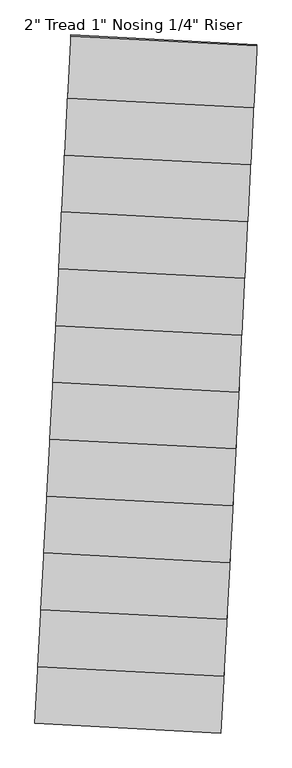
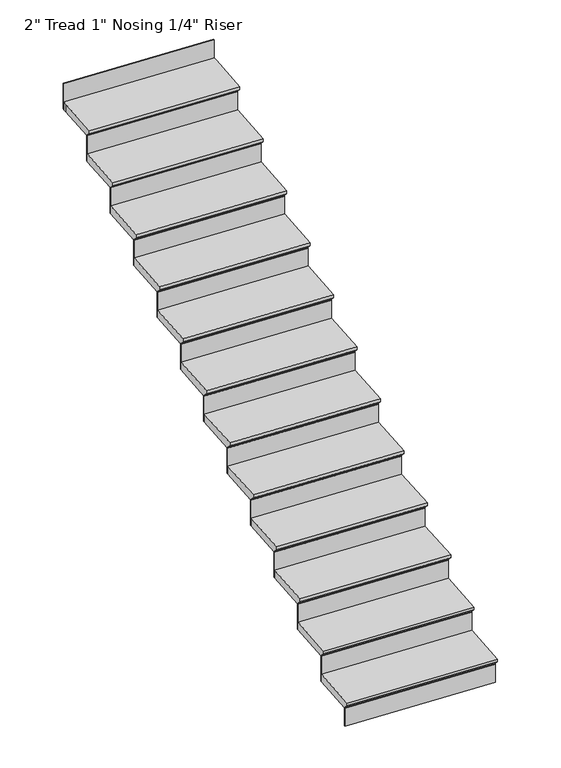
"""IFC4 building model written with IfcOpenShell, lengths in millimetres: stair flight geometry."""

from ifc_helpers import new_model, si_unit, origin, place, context, project, spatial, faceted_brep, source, transform, mapped, element, save


def stair_flight_fe3b1aa7(model_context):
    return source(origin(), model_context, "Body", "Brep", [
        faceted_brep([(-18700.9481023, 10719.3933247, 150.2833333), (-18700.9481023, 10719.3933247, 169.3333333), (-19614.0949489, 10767.2493231, 169.3333333), (-19614.0949489, 10767.2493231, 150.2833333), (-18699.618769, 10744.7585149, 124.8833333), (-19612.7656156, 10792.6145133, 124.8833333), (-18684.9961029, 11023.7756069, 169.3333333), (-19598.1429494, 11071.6316053, 169.3333333), (-19612.7656156, 10792.6145133, 118.5333333), (-19598.1429494, 11071.6316053, 118.5333333), (-18684.9961029, 11023.7756069, 118.5333333), (-18699.618769, 10744.7585149, 118.5333333)], [[[0, 1, 2, 3]], [[4, 0, 3, 5]], [[2, 1, 6, 7]], [[8, 9, 10, 11]], [[2, 7, 9, 8, 5, 3]], [[8, 11, 4, 5]], [[6, 1, 0, 4, 11, 10]], [[7, 6, 10, 9]]]),
        faceted_brep([(-18699.618769, 10744.7585149, 118.5333333), (-18699.618769, 10744.7585149, 0.0), (-18699.2864357, 10751.0998125, 0.0), (-18699.2864357, 10751.0998125, 118.5333333), (-19612.7656156, 10792.6145133, 118.5333333), (-19612.4332823, 10798.9558108, 118.5333333), (-19612.4332823, 10798.9558108, 0.0), (-19612.7656156, 10792.6145133, 0.0)], [[[0, 1, 2, 3]], [[4, 5, 6, 7]], [[1, 0, 4, 7]], [[2, 1, 7, 6]], [[3, 2, 6, 5]], [[0, 3, 5, 4]]]),
        faceted_brep([(-18684.9961029, 11023.7756069, 287.8666667), (-18684.9961029, 11023.7756069, 118.5333333), (-18684.6637695, 11030.1169045, 118.5333333), (-18684.6637695, 11030.1169045, 287.8666667), (-19598.1429494, 11071.6316053, 287.8666667), (-19597.8106161, 11077.9729029, 287.8666667), (-19597.8106161, 11077.9729029, 118.5333333), (-19598.1429494, 11071.6316053, 118.5333333)], [[[0, 1, 2, 3]], [[4, 5, 6, 7]], [[1, 0, 4, 7]], [[2, 1, 7, 6]], [[3, 2, 6, 5]], [[0, 3, 5, 4]]]),
        faceted_brep([(-19599.4722827, 11046.2664151, 338.6666667), (-18686.3254362, 10998.4104167, 338.6666667), (-18670.3734367, 11302.7926989, 338.6666667), (-19583.5202833, 11350.6486973, 338.6666667), (-19598.1429494, 11071.6316053, 287.8666667), (-19583.5202833, 11350.6486973, 287.8666667), (-18670.3734367, 11302.7926989, 287.8666667), (-18684.9961029, 11023.7756069, 287.8666667), (-19598.1429494, 11071.6316053, 294.2166667), (-19599.4722827, 11046.2664151, 319.6166667), (-18684.9961029, 11023.7756069, 294.2166667), (-18686.3254362, 10998.4104167, 319.6166667)], [[[0, 1, 2, 3]], [[4, 5, 6, 7]], [[0, 3, 5, 4, 8, 9]], [[4, 7, 10, 8]], [[2, 1, 11, 10, 7, 6]], [[3, 2, 6, 5]], [[11, 1, 0, 9]], [[10, 11, 9, 8]]]),
        faceted_brep([(-18670.3734367, 11302.7926989, 457.2), (-18670.3734367, 11302.7926989, 287.8666667), (-18670.0411034, 11309.1339965, 287.8666667), (-18670.0411034, 11309.1339965, 457.2), (-19583.5202833, 11350.6486973, 457.2), (-19583.1879499, 11356.9899949, 457.2), (-19583.1879499, 11356.9899949, 287.8666667), (-19583.5202833, 11350.6486973, 287.8666667)], [[[0, 1, 2, 3]], [[4, 5, 6, 7]], [[1, 0, 4, 7]], [[2, 1, 7, 6]], [[3, 2, 6, 5]], [[0, 3, 5, 4]]]),
        faceted_brep([(-19584.8496166, 11325.2835071, 508.0), (-18671.70277, 11277.4275087, 508.0), (-18655.7507705, 11581.8097909, 508.0), (-19568.8976171, 11629.6657893, 508.0), (-19583.5202833, 11350.6486973, 457.2), (-19568.8976171, 11629.6657893, 457.2), (-18655.7507705, 11581.8097909, 457.2), (-18670.3734367, 11302.7926989, 457.2), (-19583.5202833, 11350.6486973, 463.55), (-19584.8496166, 11325.2835071, 488.95), (-18670.3734367, 11302.7926989, 463.55), (-18671.70277, 11277.4275087, 488.95)], [[[0, 1, 2, 3]], [[4, 5, 6, 7]], [[0, 3, 5, 4, 8, 9]], [[4, 7, 10, 8]], [[2, 1, 11, 10, 7, 6]], [[3, 2, 6, 5]], [[11, 1, 0, 9]], [[10, 11, 9, 8]]]),
        faceted_brep([(-18655.7507705, 11581.8097909, 626.5333333), (-18655.7507705, 11581.8097909, 457.2), (-18655.4184372, 11588.1510885, 457.2), (-18655.4184372, 11588.1510885, 626.5333333), (-19568.8976171, 11629.6657893, 626.5333333), (-19568.5652838, 11636.0070869, 626.5333333), (-19568.5652838, 11636.0070869, 457.2), (-19568.8976171, 11629.6657893, 457.2)], [[[0, 1, 2, 3]], [[4, 5, 6, 7]], [[1, 0, 4, 7]], [[2, 1, 7, 6]], [[3, 2, 6, 5]], [[0, 3, 5, 4]]]),
        faceted_brep([(-19570.2269504, 11604.3005991, 677.3333333), (-18657.0801038, 11556.4446008, 677.3333333), (-18641.1281043, 11860.826883, 677.3333333), (-19554.2749509, 11908.6828813, 677.3333333), (-19568.8976171, 11629.6657893, 626.5333333), (-19554.2749509, 11908.6828813, 626.5333333), (-18641.1281043, 11860.826883, 626.5333333), (-18655.7507705, 11581.8097909, 626.5333333), (-19568.8976171, 11629.6657893, 632.8833333), (-19570.2269504, 11604.3005991, 658.2833333), (-18655.7507705, 11581.8097909, 632.8833333), (-18657.0801038, 11556.4446008, 658.2833333)], [[[0, 1, 2, 3]], [[4, 5, 6, 7]], [[0, 3, 5, 4, 8, 9]], [[4, 7, 10, 8]], [[2, 1, 11, 10, 7, 6]], [[3, 2, 6, 5]], [[11, 1, 0, 9]], [[10, 11, 9, 8]]]),
        faceted_brep([(-18641.1281043, 11860.826883, 795.8666667), (-18641.1281043, 11860.826883, 626.5333333), (-18640.795771, 11867.1681805, 626.5333333), (-18640.795771, 11867.1681805, 795.8666667), (-19554.2749509, 11908.6828813, 795.8666667), (-19553.9426176, 11915.0241789, 795.8666667), (-19553.9426176, 11915.0241789, 626.5333333), (-19554.2749509, 11908.6828813, 626.5333333)], [[[0, 1, 2, 3]], [[4, 5, 6, 7]], [[1, 0, 4, 7]], [[2, 1, 7, 6]], [[3, 2, 6, 5]], [[0, 3, 5, 4]]]),
        faceted_brep([(-19555.6042842, 11883.3176912, 846.6666667), (-18642.4574376, 11835.4616928, 846.6666667), (-18626.5054382, 12139.843975, 846.6666667), (-19539.6522847, 12187.6999733, 846.6666667), (-19554.2749509, 11908.6828813, 795.8666667), (-19539.6522847, 12187.6999733, 795.8666667), (-18626.5054382, 12139.843975, 795.8666667), (-18641.1281043, 11860.826883, 795.8666667), (-19554.2749509, 11908.6828813, 802.2166667), (-19555.6042842, 11883.3176912, 827.6166667), (-18641.1281043, 11860.826883, 802.2166667), (-18642.4574376, 11835.4616928, 827.6166667)], [[[0, 1, 2, 3]], [[4, 5, 6, 7]], [[0, 3, 5, 4, 8, 9]], [[4, 7, 10, 8]], [[2, 1, 11, 10, 7, 6]], [[3, 2, 6, 5]], [[11, 1, 0, 9]], [[10, 11, 9, 8]]]),
        faceted_brep([(-18626.5054382, 12139.843975, 965.2), (-18626.5054382, 12139.843975, 795.8666667), (-18626.1731048, 12146.1852725, 795.8666667), (-18626.1731048, 12146.1852725, 965.2), (-19539.6522847, 12187.6999733, 965.2), (-19539.3199514, 12194.0412709, 965.2), (-19539.3199514, 12194.0412709, 795.8666667), (-19539.6522847, 12187.6999733, 795.8666667)], [[[0, 1, 2, 3]], [[4, 5, 6, 7]], [[1, 0, 4, 7]], [[2, 1, 7, 6]], [[3, 2, 6, 5]], [[0, 3, 5, 4]]]),
        faceted_brep([(-19540.981618, 12162.3347832, 1016.0), (-18627.8347715, 12114.4787848, 1016.0), (-18611.882772, 12418.861067, 1016.0), (-19525.0296186, 12466.7170654, 1016.0), (-19539.6522847, 12187.6999733, 965.2), (-19525.0296186, 12466.7170654, 965.2), (-18611.882772, 12418.861067, 965.2), (-18626.5054382, 12139.843975, 965.2), (-19539.6522847, 12187.6999733, 971.55), (-19540.981618, 12162.3347832, 996.95), (-18626.5054382, 12139.843975, 971.55), (-18627.8347715, 12114.4787848, 996.95)], [[[0, 1, 2, 3]], [[4, 5, 6, 7]], [[0, 3, 5, 4, 8, 9]], [[4, 7, 10, 8]], [[2, 1, 11, 10, 7, 6]], [[3, 2, 6, 5]], [[11, 1, 0, 9]], [[10, 11, 9, 8]]]),
        faceted_brep([(-18611.882772, 12418.861067, 1134.5333333), (-18611.882772, 12418.861067, 965.2), (-18611.5504387, 12425.2023645, 965.2), (-18611.5504387, 12425.2023645, 1134.5333333), (-19525.0296186, 12466.7170654, 1134.5333333), (-19524.6972853, 12473.0583629, 1134.5333333), (-19524.6972853, 12473.0583629, 965.2), (-19525.0296186, 12466.7170654, 965.2)], [[[0, 1, 2, 3]], [[4, 5, 6, 7]], [[1, 0, 4, 7]], [[2, 1, 7, 6]], [[3, 2, 6, 5]], [[0, 3, 5, 4]]]),
        faceted_brep([(-19526.3589519, 12441.3518752, 1185.3333333), (-18613.2121053, 12393.4958768, 1185.3333333), (-18597.2601058, 12697.878159, 1185.3333333), (-19510.4069524, 12745.7341574, 1185.3333333), (-19525.0296186, 12466.7170654, 1134.5333333), (-19510.4069524, 12745.7341574, 1134.5333333), (-18597.2601058, 12697.878159, 1134.5333333), (-18611.882772, 12418.861067, 1134.5333333), (-19525.0296186, 12466.7170654, 1140.8833333), (-19526.3589519, 12441.3518752, 1166.2833333), (-18611.882772, 12418.861067, 1140.8833333), (-18613.2121053, 12393.4958768, 1166.2833333)], [[[0, 1, 2, 3]], [[4, 5, 6, 7]], [[0, 3, 5, 4, 8, 9]], [[4, 7, 10, 8]], [[2, 1, 11, 10, 7, 6]], [[3, 2, 6, 5]], [[11, 1, 0, 9]], [[10, 11, 9, 8]]]),
        faceted_brep([(-18597.2601058, 12697.878159, 1303.8666667), (-18597.2601058, 12697.878159, 1134.5333333), (-18596.9277725, 12704.2194565, 1134.5333333), (-18596.9277725, 12704.2194565, 1303.8666667), (-19510.4069524, 12745.7341574, 1303.8666667), (-19510.0746191, 12752.0754549, 1303.8666667), (-19510.0746191, 12752.0754549, 1134.5333333), (-19510.4069524, 12745.7341574, 1134.5333333)], [[[0, 1, 2, 3]], [[4, 5, 6, 7]], [[1, 0, 4, 7]], [[2, 1, 7, 6]], [[3, 2, 6, 5]], [[0, 3, 5, 4]]]),
        faceted_brep([(-19511.7362857, 12720.3689672, 1354.6666667), (-18598.5894391, 12672.5129688, 1354.6666667), (-18582.6374396, 12976.895251, 1354.6666667), (-19495.7842862, 13024.7512494, 1354.6666667), (-19510.4069524, 12745.7341574, 1303.8666667), (-19495.7842862, 13024.7512494, 1303.8666667), (-18582.6374396, 12976.895251, 1303.8666667), (-18597.2601058, 12697.878159, 1303.8666667), (-19510.4069524, 12745.7341574, 1310.2166667), (-19511.7362857, 12720.3689672, 1335.6166667), (-18597.2601058, 12697.878159, 1310.2166667), (-18598.5894391, 12672.5129688, 1335.6166667)], [[[0, 1, 2, 3]], [[4, 5, 6, 7]], [[0, 3, 5, 4, 8, 9]], [[4, 7, 10, 8]], [[2, 1, 11, 10, 7, 6]], [[3, 2, 6, 5]], [[11, 1, 0, 9]], [[10, 11, 9, 8]]]),
        faceted_brep([(-18582.6374396, 12976.895251, 1473.2), (-18582.6374396, 12976.895251, 1303.8666667), (-18582.3051063, 12983.2365485, 1303.8666667), (-18582.3051063, 12983.2365485, 1473.2), (-19495.7842862, 13024.7512494, 1473.2), (-19495.4519529, 13031.0925469, 1473.2), (-19495.4519529, 13031.0925469, 1303.8666667), (-19495.7842862, 13024.7512494, 1303.8666667)], [[[0, 1, 2, 3]], [[4, 5, 6, 7]], [[1, 0, 4, 7]], [[2, 1, 7, 6]], [[3, 2, 6, 5]], [[0, 3, 5, 4]]]),
        faceted_brep([(-19497.1136195, 12999.3860592, 1524.0), (-18583.9667729, 12951.5300608, 1524.0), (-18568.0147735, 13255.912343, 1524.0), (-19481.1616201, 13303.7683414, 1524.0), (-19495.7842862, 13024.7512494, 1473.2), (-19481.1616201, 13303.7683414, 1473.2), (-18568.0147735, 13255.912343, 1473.2), (-18582.6374396, 12976.895251, 1473.2), (-19495.7842862, 13024.7512494, 1479.55), (-19497.1136195, 12999.3860592, 1504.95), (-18582.6374396, 12976.895251, 1479.55), (-18583.9667729, 12951.5300608, 1504.95)], [[[0, 1, 2, 3]], [[4, 5, 6, 7]], [[0, 3, 5, 4, 8, 9]], [[4, 7, 10, 8]], [[2, 1, 11, 10, 7, 6]], [[3, 2, 6, 5]], [[11, 1, 0, 9]], [[10, 11, 9, 8]]]),
        faceted_brep([(-18568.0147735, 13255.912343, 1642.5333333), (-18568.0147735, 13255.912343, 1473.2), (-18567.6824401, 13262.2536405, 1473.2), (-18567.6824401, 13262.2536405, 1642.5333333), (-19481.1616201, 13303.7683414, 1642.5333333), (-19480.8292867, 13310.1096389, 1642.5333333), (-19480.8292867, 13310.1096389, 1473.2), (-19481.1616201, 13303.7683414, 1473.2)], [[[0, 1, 2, 3]], [[4, 5, 6, 7]], [[1, 0, 4, 7]], [[2, 1, 7, 6]], [[3, 2, 6, 5]], [[0, 3, 5, 4]]]),
        faceted_brep([(-19482.4909533, 13278.4031512, 1693.3333333), (-18569.3441068, 13230.5471528, 1693.3333333), (-18553.3921073, 13534.929435, 1693.3333333), (-19466.5389539, 13582.7854334, 1693.3333333), (-19481.1616201, 13303.7683414, 1642.5333333), (-19466.5389539, 13582.7854334, 1642.5333333), (-18553.3921073, 13534.929435, 1642.5333333), (-18568.0147735, 13255.912343, 1642.5333333), (-19481.1616201, 13303.7683414, 1648.8833333), (-19482.4909533, 13278.4031512, 1674.2833333), (-18568.0147735, 13255.912343, 1648.8833333), (-18569.3441068, 13230.5471528, 1674.2833333)], [[[0, 1, 2, 3]], [[4, 5, 6, 7]], [[0, 3, 5, 4, 8, 9]], [[4, 7, 10, 8]], [[2, 1, 11, 10, 7, 6]], [[3, 2, 6, 5]], [[11, 1, 0, 9]], [[10, 11, 9, 8]]]),
        faceted_brep([(-18553.3921073, 13534.929435, 1811.8666667), (-18553.3921073, 13534.929435, 1642.5333333), (-18553.059774, 13541.2707326, 1642.5333333), (-18553.059774, 13541.2707326, 1811.8666667), (-19466.5389539, 13582.7854334, 1811.8666667), (-19466.2066206, 13589.1267309, 1811.8666667), (-19466.2066206, 13589.1267309, 1642.5333333), (-19466.5389539, 13582.7854334, 1642.5333333)], [[[0, 1, 2, 3]], [[4, 5, 6, 7]], [[1, 0, 4, 7]], [[2, 1, 7, 6]], [[3, 2, 6, 5]], [[0, 3, 5, 4]]]),
        faceted_brep([(-19467.8682872, 13557.4202432, 1862.6666667), (-18554.7214406, 13509.5642448, 1862.6666667), (-18538.7694411, 13813.946527, 1862.6666667), (-19451.9162877, 13861.8025254, 1862.6666667), (-19466.5389539, 13582.7854334, 1811.8666667), (-19451.9162877, 13861.8025254, 1811.8666667), (-18538.7694411, 13813.946527, 1811.8666667), (-18553.3921073, 13534.929435, 1811.8666667), (-19466.5389539, 13582.7854334, 1818.2166667), (-19467.8682872, 13557.4202432, 1843.6166667), (-18553.3921073, 13534.929435, 1818.2166667), (-18554.7214406, 13509.5642448, 1843.6166667)], [[[0, 1, 2, 3]], [[4, 5, 6, 7]], [[0, 3, 5, 4, 8, 9]], [[4, 7, 10, 8]], [[2, 1, 11, 10, 7, 6]], [[3, 2, 6, 5]], [[11, 1, 0, 9]], [[10, 11, 9, 8]]]),
        faceted_brep([(-18524.1467749, 14092.963619, 2150.5333333), (-18524.1467749, 14092.963619, 1981.2), (-18523.8144416, 14099.3049166, 1981.2), (-18523.8144416, 14099.3049166, 2150.5333333), (-19437.2936215, 14140.8196174, 2150.5333333), (-19436.9612882, 14147.160915, 2150.5333333), (-19436.9612882, 14147.160915, 1981.2), (-19437.2936215, 14140.8196174, 1981.2)], [[[0, 1, 2, 3]], [[4, 5, 6, 7]], [[1, 0, 4, 7]], [[2, 1, 7, 6]], [[3, 2, 6, 5]], [[0, 3, 5, 4]]]),
        faceted_brep([(-18538.7694411, 13813.946527, 1981.2), (-18538.7694411, 13813.946527, 1811.8666667), (-18538.4371078, 13820.2878246, 1811.8666667), (-18538.4371078, 13820.2878246, 1981.2), (-19451.9162877, 13861.8025254, 1981.2), (-19451.5839544, 13868.143823, 1981.2), (-19451.5839544, 13868.143823, 1811.8666667), (-19451.9162877, 13861.8025254, 1811.8666667)], [[[0, 1, 2, 3]], [[4, 5, 6, 7]], [[1, 0, 4, 7]], [[2, 1, 7, 6]], [[3, 2, 6, 5]], [[0, 3, 5, 4]]]),
        faceted_brep([(-19437.2936215, 14140.8196174, 2032.0), (-19438.6229548, 14115.4544272, 2032.0), (-19453.245621, 13836.4373352, 2032.0), (-18540.0987744, 13788.5813368, 2032.0), (-18525.4761082, 14067.5984289, 2032.0), (-18524.1467749, 14092.963619, 2032.0), (-19438.6229548, 14115.4544272, 1981.2), (-19437.2936215, 14140.8196174, 1981.2), (-18524.1467749, 14092.963619, 1981.2), (-18525.4761082, 14067.5984289, 1981.2), (-18538.7694411, 13813.946527, 1981.2), (-19451.9162877, 13861.8025254, 1981.2), (-19451.9162877, 13861.8025254, 1987.55), (-19453.245621, 13836.4373352, 2012.95), (-18538.7694411, 13813.946527, 1987.55), (-18540.0987744, 13788.5813368, 2012.95)], [[[0, 1, 2, 3, 4, 5]], [[6, 7, 8, 9, 10, 11]], [[1, 0, 7, 6]], [[2, 1, 6, 11, 12, 13]], [[11, 10, 14, 12]], [[4, 3, 15, 14, 10, 9]], [[5, 4, 9, 8]], [[0, 5, 8, 7]], [[15, 3, 2, 13]], [[14, 15, 13, 12]]]),
    ])


if __name__ == "__main__":
    model = new_model("IFC4")
    model_context = context("Model", 3, world=origin())
    ifc_project = project(units=[si_unit("LENGTHUNIT", "METRE", prefix="MILLI")], contexts=[model_context])
    site = spatial("IfcSite", under=ifc_project)
    building = spatial("IfcBuilding", under=site)
    placement = place(None, origin())
    stair_flight_shape = stair_flight_fe3b1aa7(model_context)
    element("IfcStairFlight", 1, ObjectType="2\" Tread 1\" Nosing 1/4\" Riser", at=placement, inside=building, context=model_context, shape_type="MappedRepresentation", body=[
        mapped(stair_flight_shape, transform((0.0, 0.0, 0.0), x_axis=(1.0, 0.0, 0.0), y_axis=(0.0, 1.0, 0.0), z_axis=(0.0, 0.0, 1.0))),
    ])
    save(model, "model.ifc")
